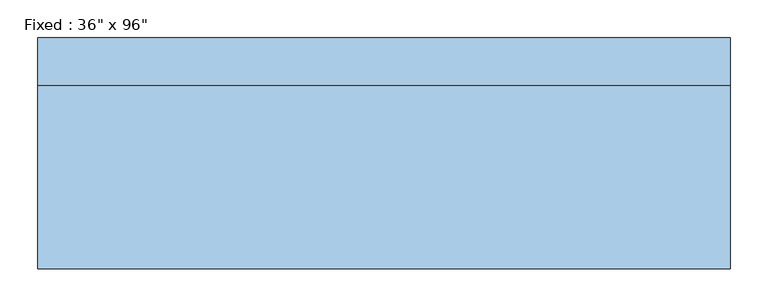
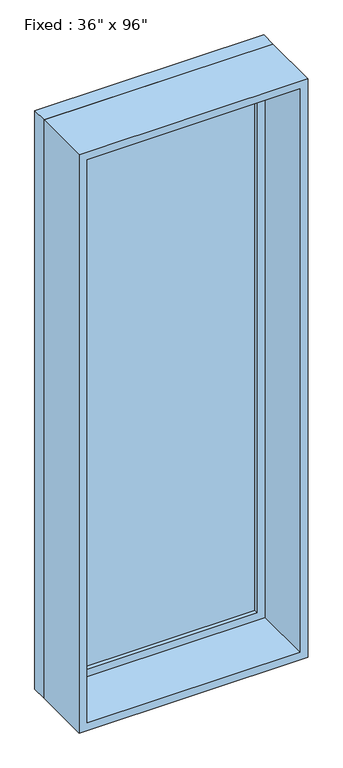
"""IFC4 building model written with IfcOpenShell, lengths in millimetres: window geometry."""

from ifc_helpers import new_model, si_unit, frame, origin, place, context, project, spatial, polyline, outline, extrude, source, transform, mapped, element, save


def window_a209d960(model_context):
    return source(origin(), model_context, "Body", "SweptSolid", [
        extrude(outline(polyline([(355.6, 104.775), (-431.8, 104.775), (-431.8, 117.475), (355.6, 117.475), (355.6, 104.775)])), frame((0.0, 0.0, 368.3), z_axis=(0.0, 0.0, 1.0), x_axis=(1.0, 0.0, 0.0)), (0.0, 0.0, 1.0), 2311.4),
        extrude(outline(polyline([(2724.15, -476.25), (323.85, -476.25), (323.85, 400.05), (2724.15, 400.05), (2724.15, -476.25)]), holes=[polyline([(2679.7, -431.8), (2679.7, 355.6), (368.3, 355.6), (368.3, -431.8), (2679.7, -431.8)])]), frame((0.0, 88.9, 0.0), z_axis=(0.0, 1.0, 0.0), x_axis=(0.0, 0.0, 1.0)), (0.0, 0.0, 1.0), 44.45),
        extrude(outline(polyline([(2743.2, -495.3), (304.8, -495.3), (304.8, 419.1), (2743.2, 419.1), (2743.2, -495.3)]), holes=[polyline([(2711.45, -463.55), (2711.45, 387.35), (336.55, 387.35), (336.55, -463.55), (2711.45, -463.55)])]), frame((0.0, -152.4, 0.0), z_axis=(0.0, 1.0, 0.0), x_axis=(0.0, 0.0, 1.0)), (0.0, 0.0, 1.0), 241.3),
        extrude(outline(polyline([(2743.2, 419.1), (2743.2, -495.3), (304.8, -495.3), (304.8, 419.1), (2743.2, 419.1)]), holes=[polyline([(2724.15, 400.05), (323.85, 400.05), (323.85, -476.25), (2724.15, -476.25), (2724.15, 400.05)])]), frame((0.0, 88.9, 0.0), z_axis=(0.0, 1.0, 0.0), x_axis=(0.0, 0.0, 1.0)), (0.0, 0.0, 1.0), 63.5),
    ])


if __name__ == "__main__":
    model = new_model("IFC4")
    model_context = context("Model", 3, world=origin())
    ifc_project = project(units=[si_unit("LENGTHUNIT", "METRE", prefix="MILLI")], contexts=[model_context])
    site = spatial("IfcSite", under=ifc_project)
    building = spatial("IfcBuilding", under=site)
    placement = place(None, origin())
    window_shape = window_a209d960(model_context)
    element("IfcWindow", 1, ObjectType="Fixed : 36\" x 96\"", at=placement, inside=building, context=model_context, shape_type="MappedRepresentation", body=[
        mapped(window_shape, transform((0.0, 0.0, 0.0), x_axis=(1.0, 0.0, 0.0), y_axis=(0.0, 1.0, 0.0), z_axis=(0.0, 0.0, 1.0))),
    ])
    save(model, "model.ifc")

# Revit data of these elements
# Type "Fixed : 36\" x 96\""
#   Type Mark = "9"
#   Construction Type Id = "GSP4R"
#   Assembly Code = "B2020100"
#   Analytic Construction = "1/8 in Pilkington single glazing"
#   Visual Light Transmittance = 0.9
#   Solar Heat Gain Coefficient = 0.78
#   Heat Transfer Coefficient (U) = 0.6496 BTU/(h·ft²·°F)
#   Height = 8' - 0"
#   Default Sill Height = 1' - 0"
#   Width = 3' - 0"
#   Window Inset = 0' - 0 3/4"
#   Define Thermal Properties by = 1
#   Glass Pane Material = Glass
#   Sash Material = Iron, Ductile
#   Wall Closure = (empty or 0)
# Element 1 (IfcWindow, "Fixed : 36\" x 96\"")
#   Materials on its faces: "Iron, Ductile", "Glass"
# Materials
#   "Glass": class "Glass", colour RGB 0 128 192, transparency 0.75, Description = "Soda Lime Glass", Cost = 0
#   "Iron, Ductile": class "Metal", colour RGB 0 0 0, transparency 0, Description = "Ductile cast iron", Cost = 0
